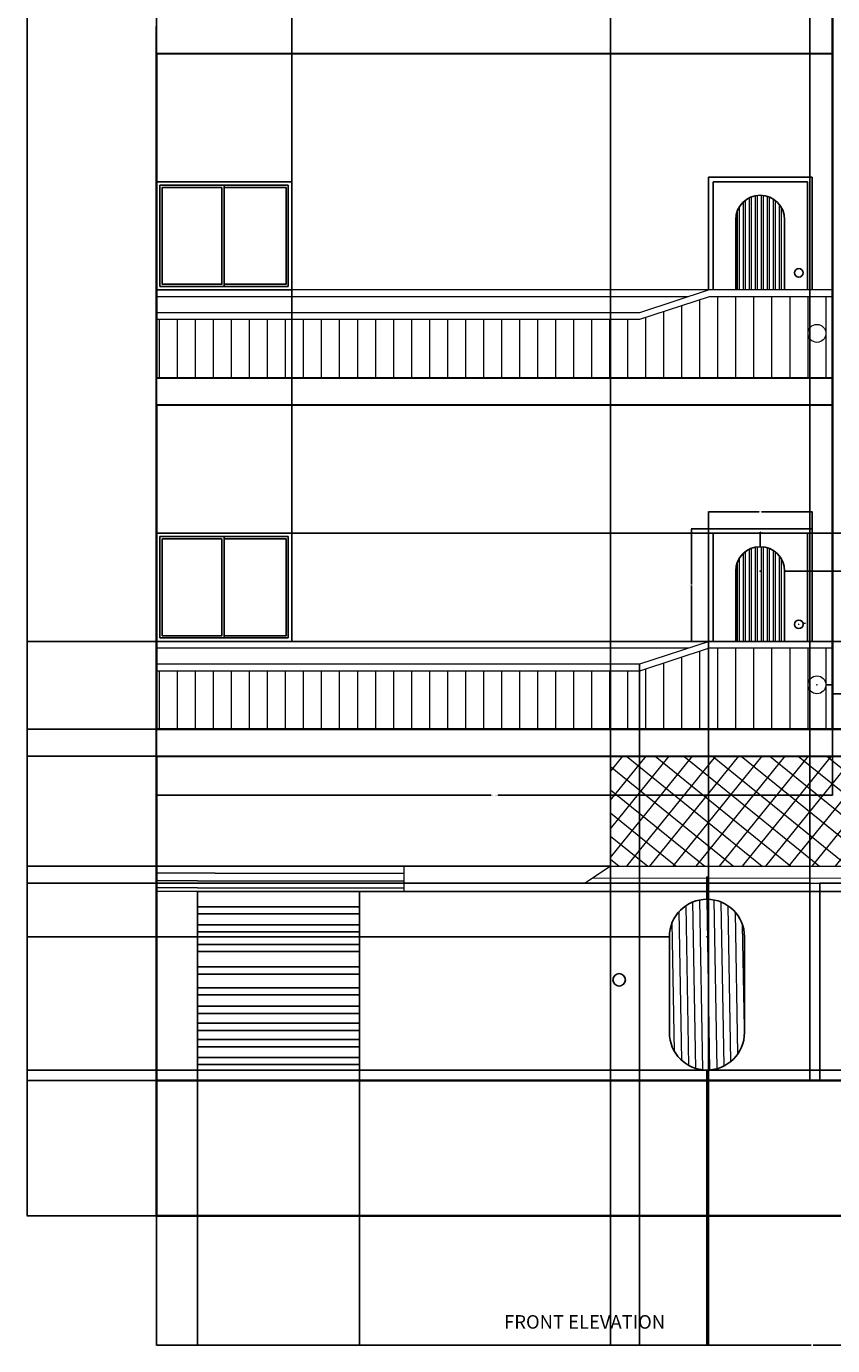
# Model space of a CAD drawing. Units: inches. Extents: x 373 to 969, y 157 to 1341.
# Tile 1 of 3: x 373 to 731, y 157 to 743. Entities that reach past the tile are written whole.
import ezdxf

# ---------------------------------------------------------------- set-up
doc = ezdxf.new("R2010")
doc.units = ezdxf.units.IN
doc.header["$MEASUREMENT"] = 0
for name, color, linetype, lineweight in [('A-ANNO-DIMS', 2, 'Continuous', 18), ('A-ANNO-TEXT', 7, 'Continuous', 25), ('A-DOOR', 3, 'Continuous', 25), ('A-DOOR-PATT', 8, 'Continuous', 13), ('A-ELEV-TRIM', 9, 'Continuous', 18), ('A-FLOR', 7, 'Continuous', 30), ('A-FLOR-HRAL', 4, 'Continuous', 18), ('A-FLOR-HRAL-PATT', 8, 'Continuous', 13), ('A-GLAZ', 4, 'Continuous', 25), ('A-WALL', 7, 'Continuous', 35), ('A-WALL-PATT', 8, 'Continuous', 13)]:
    doc.layers.add(name, color=color, linetype=linetype, lineweight=lineweight)
doc.styles.get("Standard").update_dxf_attribs({"font": 'arial.ttf'})
doc.dimstyles.get("Standard").update_dxf_attribs({"dimtxt": 0.18, "dimasz": 0.18, "dimexe": 0.18, "dimexo": 0.0625, "dimgap": 0.09, "dimtad": 0, "dimtih": 1, "dimtoh": 1, "dimdec": 4, "dimzin": 0, "dimdsep": 46, "dimlunit": 4, "dimtxsty": 'Standard', "dimcen": 0.09, "dimadec": 0, "dimazin": 0, "dimtfac": 1, "dimtdec": 4, "dimtofl": 0, "dimtmove": 0, "dimatfit": 3, "dimfxl": 1, "dimtolj": 1, "dimtzin": 0, "dimarcsym": 0})

# ---------------------------------------------------------------- blocks, each defined once
blk = doc.blocks.new('*U2')
for p, q in [((1.5, 1.5), (1.5, 46.5)), ((1.5, 46.5), (30, 46.5)), ((30, 1.5), (30, 46.5)), ((30, 46.5), (58.5, 46.5)), ((58.5, 46.5), (58.5, 1.5)), ((30, 1.5), (1.5, 1.5)), ((58.5, 1.5), (30, 1.5))]:
    blk.add_line(p, q)
blk.add_lwpolyline([(0, 0), (0, 48), (60, 48), (60, 0)], close=True)
for points in [[(29, 45.5), (29, 2.5), (2.5, 2.5), (2.5, 45.5), (29, 45.5)], [(30, 45.5), (57.5, 45.5), (57.5, 2.5), (30, 2.5)]]:
    blk.add_lwpolyline(points)
blk = doc.blocks.new('DOOR-ARCH-PANEL-ELEV')
for p, q in [((0, 48), (0, 50)), ((0, 50), (2, 50)), ((0, 48), (0, 0)), ((44, 50), (2, 50)), ((44, 48), (2, 48)), ((2, 48), (2, 0)), ((44, 50), (46, 50)), ((44, 0), (44, 48)), ((46, 50), (46, 48)), ((46, 0), (46, 48))]:
    blk.add_line(p, q)
for points in [[(12.07, 0), (12.07, 31.15)], [(33.78, 31.15), (33.78, 0)]]:
    blk.add_lwpolyline(points)
blk.add_circle((40.06, 7.56), 1.92)
blk.add_arc((22.93, 31.15), 10.86, 0, 180)
blk = doc.blocks.new('RAIL-BALCONY-SLOPED-ELEV')
for p, q in [((245.4, 23.26), (0, 23.26)), ((236.25, 20.26), (0, 20.26)), ((245.4, 23.26), (214.4, 13.09)), ((245.4, 20.26), (214.4, 10.09)), ((300.23, 23.26), (245.4, 23.26)), ((300.23, 20.26), (245.4, 20.26)), ((214.4, 13.09), (0, 13.09)), ((214.4, 10.09), (0, 10.09))]:
    blk.add_line(p, q)
blk.add_circle((293.27, 3.97), 3.97)
blk = doc.blocks.new('DOOR-OBROUND-INSERT-ELEV')
for points in [[(0, 16.68), (0, 59.13)], [(33.36, 59.13), (33.36, 16.68)]]:
    blk.add_lwpolyline(points)
for centre, start, end in [((16.68, 59.13), 0, 180), ((16.68, 16.68), 180, 0)]:
    blk.add_arc(centre, 16.68, start, end)
blk = doc.blocks.new('*D9')
at = {"layer": 'A-ANNO-DIMS', "color": 0, "lineweight": -2, "transparency": 16777216}
for p, q in [((675.76, 519.98), (668.14, 519.98)), ((668.32, 519.8), (668.32, 495.17)), ((668.32, 470.16), (668.32, 494.8)), ((675.76, 469.98), (668.14, 469.98))]:
    blk.add_line(p, q, dxfattribs=at)
at = {"layer": 'A-ANNO-DIMS', "color": 0, "transparency": 16777216}
for points in [[(668.29, 519.8), (668.35, 519.8), (668.32, 519.98)], [(668.29, 470.16), (668.35, 470.16), (668.32, 469.98)]]:
    blk.add_solid(points, dxfattribs=at)
at = {"layer": 'Defpoints', "color": 0, "transparency": 16777216}
for p in [(668.32, 519.98), (675.82, 519.98), (675.82, 469.98)]:
    blk.add_point(p, dxfattribs=at)
at = {"layer": 'A-ANNO-DIMS', "color": 0, "transparency": 16777216, "insert": (668.32, 494.98), "char_height": 0.18, "attachment_point": 5}
blk.add_mtext('\\A1;ARCH DOOR 50 TYP.', dxfattribs=at)
blk = doc.blocks.new('*D10')
at = {"layer": 'A-ANNO-DIMS', "color": 0, "lineweight": -2, "transparency": 16777216}
for p, q in [((675.82, 520.05), (675.82, 527.66)), ((676, 527.48), (698.29, 527.48)), ((721.64, 527.48), (699.36, 527.48)), ((721.82, 520.05), (721.82, 527.66))]:
    blk.add_line(p, q, dxfattribs=at)
at = {"layer": 'A-ANNO-DIMS', "color": 0, "transparency": 16777216}
for points in [[(676, 527.51), (676, 527.45), (675.82, 527.48)], [(721.64, 527.51), (721.64, 527.45), (721.82, 527.48)]]:
    blk.add_solid(points, dxfattribs=at)
at = {"layer": 'Defpoints', "color": 0, "transparency": 16777216}
for p in [(721.82, 527.48), (675.82, 519.98), (721.82, 519.98)]:
    blk.add_point(p, dxfattribs=at)
at = {"layer": 'A-ANNO-DIMS', "color": 0, "transparency": 16777216, "insert": (698.82, 527.48), "char_height": 0.18, "attachment_point": 5}
blk.add_mtext('\\A1;46 TYP.', dxfattribs=at)
blk = doc.blocks.new('*D11')
at = {"layer": 'A-ANNO-DIMS', "color": 0, "lineweight": -2, "transparency": 16777216}
for p, q in [((430.7, 446.66), (430.7, 401.51)), ((730.93, 446.66), (730.93, 401.51)), ((430.88, 401.69), (579.36, 401.69)), ((730.75, 401.69), (582.27, 401.69))]:
    blk.add_line(p, q, dxfattribs=at)
at = {"layer": 'A-ANNO-DIMS', "color": 0, "transparency": 16777216}
for points in [[(430.88, 401.72), (430.88, 401.66), (430.7, 401.69)], [(730.75, 401.72), (730.75, 401.66), (730.93, 401.69)]]:
    blk.add_solid(points, dxfattribs=at)
at = {"layer": 'Defpoints', "color": 0, "transparency": 16777216}
for p in [(430.7, 446.72), (730.93, 446.72), (730.93, 401.69)]:
    blk.add_point(p, dxfattribs=at)
at = {"layer": 'A-ANNO-DIMS', "color": 0, "transparency": 16777216, "insert": (580.82, 401.69), "char_height": 0.18, "attachment_point": 5}
blk.add_mtext('\\A1;SLOPED RAIL 300 TYP.', dxfattribs=at)
blk = doc.blocks.new('*D12')
at = {"layer": 'A-ANNO-DIMS', "color": 0, "lineweight": -2, "transparency": 16777216}
for p, q in [((731, 469.98), (776.15, 469.98)), ((775.97, 469.8), (775.97, 458.53)), ((775.97, 446.9), (775.97, 458.17)), ((731, 446.72), (776.15, 446.72))]:
    blk.add_line(p, q, dxfattribs=at)
at = {"layer": 'A-ANNO-DIMS', "color": 0, "transparency": 16777216}
for points in [[(775.94, 469.8), (776, 469.8), (775.97, 469.98)], [(775.94, 446.9), (776, 446.9), (775.97, 446.72)]]:
    blk.add_solid(points, dxfattribs=at)
at = {"layer": 'Defpoints', "color": 0, "transparency": 16777216}
for p in [(730.93, 469.98), (775.97, 469.98), (730.93, 446.72)]:
    blk.add_point(p, dxfattribs=at)
at = {"layer": 'A-ANNO-DIMS', "color": 0, "transparency": 16777216, "insert": (775.97, 458.35), "char_height": 0.18, "attachment_point": 5}
blk.add_mtext('\\A1;23 TYP.', dxfattribs=at)
blk = doc.blocks.new('*D27')
at = {"layer": 'A-ANNO-DIMS', "color": 0, "lineweight": -2, "transparency": 16777216}
for p, q in [((430.64, 469.98), (373.07, 469.98)), ((373.25, 469.8), (373.25, 450.67)), ((373.25, 431.16), (373.25, 450.3)), ((430.64, 430.98), (373.07, 430.98))]:
    blk.add_line(p, q, dxfattribs=at)
at = {"layer": 'A-ANNO-DIMS', "color": 0, "transparency": 16777216}
for points in [[(373.22, 469.8), (373.28, 469.8), (373.25, 469.98)], [(373.22, 431.16), (373.28, 431.16), (373.25, 430.98)]]:
    blk.add_solid(points, dxfattribs=at)
at = {"layer": 'Defpoints', "color": 0, "transparency": 16777216}
for p in [(373.25, 469.98), (430.7, 469.98), (430.7, 430.98)]:
    blk.add_point(p, dxfattribs=at)
at = {"layer": 'A-ANNO-DIMS', "color": 0, "transparency": 16777216, "insert": (373.25, 450.48), "char_height": 0.18, "attachment_point": 5}
blk.add_mtext('\\A1;39', dxfattribs=at)
blk = doc.blocks.new('*D28')
at = {"layer": 'A-ANNO-DIMS', "color": 0, "lineweight": -2, "transparency": 16777216}
for p, q in [((430.64, 430.98), (373.07, 430.98)), ((373.25, 430.8), (373.25, 425.16)), ((373.25, 419.16), (373.25, 424.8)), ((430.64, 418.98), (373.07, 418.98))]:
    blk.add_line(p, q, dxfattribs=at)
at = {"layer": 'A-ANNO-DIMS', "color": 0, "transparency": 16777216}
for points in [[(373.22, 430.8), (373.28, 430.8), (373.25, 430.98)], [(373.22, 419.16), (373.28, 419.16), (373.25, 418.98)]]:
    blk.add_solid(points, dxfattribs=at)
at = {"layer": 'Defpoints', "color": 0, "transparency": 16777216}
for p in [(373.25, 430.98), (430.7, 430.98), (430.7, 418.98)]:
    blk.add_point(p, dxfattribs=at)
at = {"layer": 'A-ANNO-DIMS', "color": 0, "transparency": 16777216, "insert": (373.25, 424.98), "char_height": 0.18, "attachment_point": 5}
blk.add_mtext('\\A1;12', dxfattribs=at)
blk = doc.blocks.new('*D29')
at = {"layer": 'A-ANNO-DIMS', "color": 0, "lineweight": -2, "transparency": 16777216}
for p, q in [((430.7, 518.05), (430.7, 1341.24)), ((490.7, 518.05), (490.7, 1341.24)), ((430.88, 1341.06), (460.48, 1341.06)), ((490.52, 1341.06), (460.92, 1341.06))]:
    blk.add_line(p, q, dxfattribs=at)
at = {"layer": 'A-ANNO-DIMS', "color": 0, "transparency": 16777216}
for points in [[(430.88, 1341.09), (430.88, 1341.03), (430.7, 1341.06)], [(490.52, 1341.09), (490.52, 1341.03), (490.7, 1341.06)]]:
    blk.add_solid(points, dxfattribs=at)
at = {"layer": 'Defpoints', "color": 0, "transparency": 16777216}
for p in [(490.7, 1341.06), (430.7, 517.98), (490.7, 517.98)]:
    blk.add_point(p, dxfattribs=at)
at = {"layer": 'A-ANNO-DIMS', "color": 0, "transparency": 16777216, "insert": (460.7, 1341.06), "char_height": 0.18, "attachment_point": 5}
blk.add_mtext('\\A1;60', dxfattribs=at)
blk = doc.blocks.new('*D30')
at = {"layer": 'A-ANNO-DIMS', "color": 0, "lineweight": -2, "transparency": 16777216}
for p, q in [((490.76, 517.98), (968.33, 517.98)), ((968.15, 517.8), (968.15, 494.17)), ((968.15, 470.16), (968.15, 493.8)), ((490.76, 469.98), (968.33, 469.98))]:
    blk.add_line(p, q, dxfattribs=at)
at = {"layer": 'A-ANNO-DIMS', "color": 0, "transparency": 16777216}
for points in [[(968.12, 517.8), (968.18, 517.8), (968.15, 517.98)], [(968.12, 470.16), (968.18, 470.16), (968.15, 469.98)]]:
    blk.add_solid(points, dxfattribs=at)
at = {"layer": 'Defpoints', "color": 0, "transparency": 16777216}
for p in [(490.7, 517.98), (968.15, 517.98), (490.7, 469.98)]:
    blk.add_point(p, dxfattribs=at)
at = {"layer": 'A-ANNO-DIMS', "color": 0, "transparency": 16777216, "insert": (968.15, 493.98), "char_height": 0.18, "attachment_point": 5}
blk.add_mtext('\\A1;48', dxfattribs=at)
blk = doc.blocks.new('*D31')
at = {"layer": 'A-ANNO-DIMS', "color": 0, "lineweight": -2, "transparency": 16777216}
for p, q in [((430.7, 459.75), (430.7, 157.35)), ((645.1, 459.75), (645.1, 157.35)), ((430.88, 157.53), (537.5, 157.53)), ((644.92, 157.53), (538.29, 157.53))]:
    blk.add_line(p, q, dxfattribs=at)
at = {"layer": 'A-ANNO-DIMS', "color": 0, "transparency": 16777216}
for points in [[(430.88, 157.56), (430.88, 157.5), (430.7, 157.53)], [(644.92, 157.56), (644.92, 157.5), (645.1, 157.53)]]:
    blk.add_solid(points, dxfattribs=at)
at = {"layer": 'Defpoints', "color": 0, "transparency": 16777216}
for p in [(430.7, 459.81), (645.1, 459.81), (645.1, 157.53)]:
    blk.add_point(p, dxfattribs=at)
at = {"layer": 'A-ANNO-DIMS', "color": 0, "transparency": 16777216, "insert": (537.9, 157.53), "char_height": 0.18, "attachment_point": 5}
blk.add_mtext('\\A1;214.4', dxfattribs=at)
blk = doc.blocks.new('*D32')
at = {"layer": 'A-ANNO-DIMS', "color": 0, "lineweight": -2, "transparency": 16777216}
for p, q in [((675.82, 469.92), (675.82, 157.35)), ((645.1, 459.75), (645.1, 157.35)), ((645.28, 157.53), (660, 157.53)), ((675.64, 157.53), (660.92, 157.53))]:
    blk.add_line(p, q, dxfattribs=at)
at = {"layer": 'A-ANNO-DIMS', "color": 0, "transparency": 16777216}
for points in [[(645.28, 157.56), (645.28, 157.5), (645.1, 157.53)], [(675.64, 157.56), (675.64, 157.5), (675.82, 157.53)]]:
    blk.add_solid(points, dxfattribs=at)
at = {"layer": 'Defpoints', "color": 0, "transparency": 16777216}
for p in [(675.82, 469.98), (645.1, 459.81), (675.82, 157.53)]:
    blk.add_point(p, dxfattribs=at)
at = {"layer": 'A-ANNO-DIMS', "color": 0, "transparency": 16777216, "insert": (660.46, 157.53), "char_height": 0.18, "attachment_point": 5}
blk.add_mtext('\\A1;30.726', dxfattribs=at)
blk = doc.blocks.new('*D33')
at = {"layer": 'A-ANNO-DIMS', "color": 0, "lineweight": -2, "transparency": 16777216}
for p, q in [((430.7, 274.92), (430.7, 157.35)), ((448.8, 274.92), (448.8, 157.35)), ((430.88, 157.53), (439.3, 157.53)), ((448.62, 157.53), (440.21, 157.53))]:
    blk.add_line(p, q, dxfattribs=at)
at = {"layer": 'A-ANNO-DIMS', "color": 0, "transparency": 16777216}
for points in [[(430.88, 157.56), (430.88, 157.5), (430.7, 157.53)], [(448.62, 157.56), (448.62, 157.5), (448.8, 157.53)]]:
    blk.add_solid(points, dxfattribs=at)
at = {"layer": 'Defpoints', "color": 0, "transparency": 16777216}
for p in [(430.7, 274.98), (448.8, 274.98), (448.8, 157.53)]:
    blk.add_point(p, dxfattribs=at)
at = {"layer": 'A-ANNO-DIMS', "color": 0, "transparency": 16777216, "insert": (439.75, 157.53), "char_height": 0.18, "attachment_point": 5}
blk.add_mtext('\\A1;18.103', dxfattribs=at)
blk = doc.blocks.new('*D34')
at = {"layer": 'A-ANNO-DIMS', "color": 0, "lineweight": -2, "transparency": 16777216}
for p, q in [((448.8, 274.92), (448.8, 157.35)), ((520.8, 274.92), (520.8, 157.35)), ((448.98, 157.53), (484.59, 157.53)), ((520.62, 157.53), (485.02, 157.53))]:
    blk.add_line(p, q, dxfattribs=at)
at = {"layer": 'A-ANNO-DIMS', "color": 0, "transparency": 16777216}
for points in [[(448.98, 157.56), (448.98, 157.5), (448.8, 157.53)], [(520.62, 157.56), (520.62, 157.5), (520.8, 157.53)]]:
    blk.add_solid(points, dxfattribs=at)
at = {"layer": 'Defpoints', "color": 0, "transparency": 16777216}
for p in [(448.8, 274.98), (520.8, 274.98), (520.8, 157.53)]:
    blk.add_point(p, dxfattribs=at)
at = {"layer": 'A-ANNO-DIMS', "color": 0, "transparency": 16777216, "insert": (484.8, 157.53), "char_height": 0.18, "attachment_point": 5}
blk.add_mtext('\\A1;72', dxfattribs=at)
blk = doc.blocks.new('*D35')
at = {"layer": 'A-ANNO-DIMS', "color": 0, "lineweight": -2, "transparency": 16777216}
for p, q in [((520.86, 358.98), (968.33, 358.98)), ((968.15, 358.8), (968.15, 317.17)), ((968.15, 275.16), (968.15, 316.8)), ((520.86, 274.98), (968.33, 274.98))]:
    blk.add_line(p, q, dxfattribs=at)
at = {"layer": 'A-ANNO-DIMS', "color": 0, "transparency": 16777216}
for points in [[(968.12, 358.8), (968.18, 358.8), (968.15, 358.98)], [(968.12, 275.16), (968.18, 275.16), (968.15, 274.98)]]:
    blk.add_solid(points, dxfattribs=at)
at = {"layer": 'Defpoints', "color": 0, "transparency": 16777216}
for p in [(520.8, 358.98), (968.15, 358.98), (520.8, 274.98)]:
    blk.add_point(p, dxfattribs=at)
at = {"layer": 'A-ANNO-DIMS', "color": 0, "transparency": 16777216, "insert": (968.15, 316.98), "char_height": 0.18, "attachment_point": 5}
blk.add_mtext('\\A1;84', dxfattribs=at)
blk = doc.blocks.new('*D36')
at = {"layer": 'A-ANNO-DIMS', "color": 0, "lineweight": -2, "transparency": 16777216}
for p, q in [((520.8, 274.92), (520.8, 157.35)), ((632.3, 274.92), (632.3, 157.35)), ((520.98, 157.53), (576.17, 157.53)), ((632.12, 157.53), (576.94, 157.53))]:
    blk.add_line(p, q, dxfattribs=at)
at = {"layer": 'A-ANNO-DIMS', "color": 0, "transparency": 16777216}
for points in [[(520.98, 157.56), (520.98, 157.5), (520.8, 157.53)], [(632.12, 157.56), (632.12, 157.5), (632.3, 157.53)]]:
    blk.add_solid(points, dxfattribs=at)
at = {"layer": 'Defpoints', "color": 0, "transparency": 16777216}
for p in [(520.8, 274.98), (632.3, 274.98), (632.3, 157.53)]:
    blk.add_point(p, dxfattribs=at)
at = {"layer": 'A-ANNO-DIMS', "color": 0, "transparency": 16777216, "insert": (576.55, 157.53), "char_height": 0.18, "attachment_point": 5}
blk.add_mtext('\\A1;111.5', dxfattribs=at)
blk = doc.blocks.new('*D37')
at = {"layer": 'A-ANNO-DIMS', "color": 0, "lineweight": -2, "transparency": 16777216}
for p, q in [((632.24, 362.6), (373.07, 362.6)), ((373.25, 362.42), (373.25, 318.98)), ((373.25, 275.16), (373.25, 318.61)), ((632.24, 274.98), (373.07, 274.98))]:
    blk.add_line(p, q, dxfattribs=at)
at = {"layer": 'A-ANNO-DIMS', "color": 0, "transparency": 16777216}
for points in [[(373.22, 362.42), (373.28, 362.42), (373.25, 362.6)], [(373.22, 275.16), (373.28, 275.16), (373.25, 274.98)]]:
    blk.add_solid(points, dxfattribs=at)
at = {"layer": 'Defpoints', "color": 0, "transparency": 16777216}
for p in [(373.25, 362.6), (632.3, 362.6), (632.3, 274.98)]:
    blk.add_point(p, dxfattribs=at)
at = {"layer": 'A-ANNO-DIMS', "color": 0, "transparency": 16777216, "insert": (373.25, 318.79), "char_height": 0.18, "attachment_point": 5}
blk.add_mtext('\\A1;87.62', dxfattribs=at)
blk = doc.blocks.new('*D38')
at = {"layer": 'A-ANNO-DIMS', "color": 0, "lineweight": -2, "transparency": 16777216}
for p, q in [((632.26, 418.98), (373.07, 418.98)), ((373.25, 418.8), (373.25, 394.78)), ((373.25, 370.39), (373.25, 394.41)), ((632.26, 370.21), (373.07, 370.21))]:
    blk.add_line(p, q, dxfattribs=at)
at = {"layer": 'A-ANNO-DIMS', "color": 0, "transparency": 16777216}
for points in [[(373.22, 418.8), (373.28, 418.8), (373.25, 418.98)], [(373.22, 370.39), (373.28, 370.39), (373.25, 370.21)]]:
    blk.add_solid(points, dxfattribs=at)
at = {"layer": 'Defpoints', "color": 0, "transparency": 16777216}
for p in [(373.25, 418.98), (632.32, 418.98), (632.32, 370.21)]:
    blk.add_point(p, dxfattribs=at)
at = {"layer": 'A-ANNO-DIMS', "color": 0, "transparency": 16777216, "insert": (373.25, 394.6), "char_height": 0.18, "attachment_point": 5}
blk.add_mtext('\\A1;48.78', dxfattribs=at)
blk = doc.blocks.new('*D39')
at = {"layer": 'A-ANNO-DIMS', "color": 0, "lineweight": -2, "transparency": 16777216}
for p, q in [((675.1, 279.62), (675.1, 157.35)), ((632.3, 274.92), (632.3, 157.35)), ((632.48, 157.53), (653.37, 157.53)), ((674.92, 157.53), (654.03, 157.53))]:
    blk.add_line(p, q, dxfattribs=at)
at = {"layer": 'A-ANNO-DIMS', "color": 0, "transparency": 16777216}
for points in [[(632.48, 157.56), (632.48, 157.5), (632.3, 157.53)], [(674.92, 157.56), (674.92, 157.5), (675.1, 157.53)]]:
    blk.add_solid(points, dxfattribs=at)
at = {"layer": 'Defpoints', "color": 0, "transparency": 16777216}
for p in [(675.1, 279.69), (632.3, 274.98), (675.1, 157.53)]:
    blk.add_point(p, dxfattribs=at)
at = {"layer": 'A-ANNO-DIMS', "color": 0, "transparency": 16777216, "insert": (653.7, 157.53), "char_height": 0.18, "attachment_point": 5}
blk.add_mtext('\\A1;42.8', dxfattribs=at)
blk = doc.blocks.new('*D40')
at = {"layer": 'A-ANNO-DIMS', "color": 0, "lineweight": -2, "transparency": 16777216}
for p, q in [((675.1, 279.62), (675.1, 157.35)), ((768.63, 279.62), (768.63, 157.35)), ((675.28, 157.53), (721.47, 157.53)), ((768.45, 157.53), (722.26, 157.53))]:
    blk.add_line(p, q, dxfattribs=at)
at = {"layer": 'A-ANNO-DIMS', "color": 0, "transparency": 16777216}
for points in [[(675.28, 157.56), (675.28, 157.5), (675.1, 157.53)], [(768.45, 157.56), (768.45, 157.5), (768.63, 157.53)]]:
    blk.add_solid(points, dxfattribs=at)
at = {"layer": 'Defpoints', "color": 0, "transparency": 16777216}
for p in [(675.1, 279.69), (768.63, 279.69), (768.63, 157.53)]:
    blk.add_point(p, dxfattribs=at)
at = {"layer": 'A-ANNO-DIMS', "color": 0, "transparency": 16777216, "insert": (721.86, 157.53), "char_height": 0.18, "attachment_point": 5}
blk.add_mtext('\\A1;93.53', dxfattribs=at)
blk = doc.blocks.new('*D42')
at = {"layer": 'A-ANNO-DIMS', "color": 0, "lineweight": -2, "transparency": 16777216}
for p, q in [((632.3, 362.67), (632.3, 1341.24)), ((720.88, 362.67), (720.88, 1341.24)), ((632.48, 1341.06), (676.2, 1341.06)), ((720.7, 1341.06), (676.98, 1341.06))]:
    blk.add_line(p, q, dxfattribs=at)
at = {"layer": 'A-ANNO-DIMS', "color": 0, "transparency": 16777216}
for points in [[(632.48, 1341.09), (632.48, 1341.03), (632.3, 1341.06)], [(720.7, 1341.09), (720.7, 1341.03), (720.88, 1341.06)]]:
    blk.add_solid(points, dxfattribs=at)
at = {"layer": 'Defpoints', "color": 0, "transparency": 16777216}
for p in [(720.88, 1341.06), (632.3, 362.6), (720.88, 362.6)]:
    blk.add_point(p, dxfattribs=at)
at = {"layer": 'A-ANNO-DIMS', "color": 0, "transparency": 16777216, "insert": (676.59, 1341.06), "char_height": 0.18, "attachment_point": 5}
blk.add_mtext('\\A1;88.58', dxfattribs=at)
blk = doc.blocks.new('*D43')
at = {"layer": 'A-ANNO-DIMS', "color": 0, "lineweight": -2, "transparency": 16777216}
for p, q in [((658.36, 338.82), (373.07, 338.82)), ((373.25, 338.64), (373.25, 309.43)), ((373.25, 279.87), (373.25, 309.07)), ((675.03, 279.69), (373.07, 279.69))]:
    blk.add_line(p, q, dxfattribs=at)
at = {"layer": 'A-ANNO-DIMS', "color": 0, "transparency": 16777216}
for points in [[(373.22, 338.64), (373.28, 338.64), (373.25, 338.82)], [(373.22, 279.87), (373.28, 279.87), (373.25, 279.69)]]:
    blk.add_solid(points, dxfattribs=at)
at = {"layer": 'Defpoints', "color": 0, "transparency": 16777216}
for p in [(373.25, 338.82), (658.42, 338.82), (675.1, 279.69)]:
    blk.add_point(p, dxfattribs=at)
at = {"layer": 'A-ANNO-DIMS', "color": 0, "transparency": 16777216, "insert": (373.25, 309.25), "char_height": 0.18, "attachment_point": 5}
blk.add_mtext('\\A1;59.13', dxfattribs=at)
blk = doc.blocks.new('*D44')
at = {"layer": 'A-ANNO-DIMS', "color": 0, "lineweight": -2, "transparency": 16777216}
for p, q in [((860.91, 279.69), (373.07, 279.69)), ((373.25, 279.51), (373.25, 277.52)), ((373.25, 275.16), (373.25, 277.15)), ((818.75, 274.98), (373.07, 274.98))]:
    blk.add_line(p, q, dxfattribs=at)
at = {"layer": 'A-ANNO-DIMS', "color": 0, "transparency": 16777216}
for points in [[(373.22, 279.51), (373.28, 279.51), (373.25, 279.69)], [(373.22, 275.16), (373.28, 275.16), (373.25, 274.98)]]:
    blk.add_solid(points, dxfattribs=at)
at = {"layer": 'Defpoints', "color": 0, "transparency": 16777216}
for p in [(373.25, 279.69), (860.97, 279.69), (818.82, 274.98)]:
    blk.add_point(p, dxfattribs=at)
at = {"layer": 'A-ANNO-DIMS', "color": 0, "transparency": 16777216, "insert": (373.25, 277.34), "char_height": 0.18, "attachment_point": 5}
blk.add_mtext('\\A1;4.702', dxfattribs=at)
blk = doc.blocks.new('*D45')
at = {"layer": 'A-ANNO-DIMS', "color": 0, "lineweight": -2, "transparency": 16777216}
for p, q in [((709.67, 501.13), (968.33, 501.13)), ((968.15, 500.95), (968.15, 485.74)), ((968.15, 470.16), (968.15, 485.38)), ((721.89, 469.98), (968.33, 469.98))]:
    blk.add_line(p, q, dxfattribs=at)
at = {"layer": 'A-ANNO-DIMS', "color": 0, "transparency": 16777216}
for points in [[(968.12, 500.95), (968.18, 500.95), (968.15, 501.13)], [(968.12, 470.16), (968.18, 470.16), (968.15, 469.98)]]:
    blk.add_solid(points, dxfattribs=at)
at = {"layer": 'Defpoints', "color": 0, "transparency": 16777216}
for p in [(709.61, 501.13), (968.15, 501.13), (721.82, 469.98)]:
    blk.add_point(p, dxfattribs=at)
at = {"layer": 'A-ANNO-DIMS', "color": 0, "transparency": 16777216, "insert": (968.15, 485.56), "char_height": 0.18, "attachment_point": 5}
blk.add_mtext('\\A1;31.146', dxfattribs=at)
blk = doc.blocks.new('*D55')
at = {"layer": 'A-ANNO-DIMS', "color": 0, "lineweight": -2, "transparency": 16777216}
for p, q in [((734.58, 1283.61), (373.07, 1283.61)), ((373.25, 1283.43), (373.25, 749.48)), ((373.25, 215.16), (373.25, 749.11)), ((430.64, 214.98), (373.07, 214.98))]:
    blk.add_line(p, q, dxfattribs=at)
at = {"layer": 'A-ANNO-DIMS', "color": 0, "transparency": 16777216}
for points in [[(373.22, 1283.43), (373.28, 1283.43), (373.25, 1283.61)], [(373.22, 215.16), (373.28, 215.16), (373.25, 214.98)]]:
    blk.add_solid(points, dxfattribs=at)
at = {"layer": 'Defpoints', "color": 0, "transparency": 16777216}
for p in [(373.25, 1283.61), (734.64, 1283.61), (430.7, 214.98)]:
    blk.add_point(p, dxfattribs=at)
at = {"layer": 'A-ANNO-DIMS', "color": 0, "transparency": 16777216, "insert": (373.25, 749.3), "char_height": 0.18, "attachment_point": 5}
blk.add_mtext('\\A1;1068.6', dxfattribs=at)
blk = doc.blocks.new('*D56')
at = {"layer": 'A-ANNO-DIMS', "color": 0, "lineweight": -2, "transparency": 16777216}
for p, q in [((675.28, 365.5), (675.1, 365.5)), ((675.1, 365.5), (675.1, 355.67)), ((675.01, 338.82), (675.19, 338.82)), ((675.1, 338.73), (675.1, 338.91))]:
    blk.add_line(p, q, dxfattribs=at)
at = {"layer": 'A-ANNO-DIMS', "color": 0, "transparency": 16777216}
blk.add_solid([(675.07, 355.67), (675.13, 355.67), (675.1, 355.49)], dxfattribs=at)
at = {"layer": 'Defpoints', "color": 0, "transparency": 16777216}
for p in [(675.1, 355.49), (675.1, 338.82)]:
    blk.add_point(p, dxfattribs=at)
at = {"layer": 'A-ANNO-DIMS', "color": 0, "transparency": 16777216, "insert": (676.02, 365.5), "char_height": 0.18, "attachment_point": 5}
blk.add_mtext('\\A1;6X R16.678', dxfattribs=at)
blk = doc.blocks.new('*D57')
at = {"layer": 'A-ANNO-DIMS', "color": 0, "lineweight": -2, "transparency": 16777216}
for p, q in [((698.93, 518.5), (698.75, 518.5)), ((698.75, 518.5), (698.75, 512.17)), ((698.66, 501.13), (698.84, 501.13)), ((698.75, 501.04), (698.75, 501.22))]:
    blk.add_line(p, q, dxfattribs=at)
at = {"layer": 'A-ANNO-DIMS', "color": 0, "transparency": 16777216}
blk.add_solid([(698.72, 512.17), (698.78, 512.17), (698.75, 511.99)], dxfattribs=at)
at = {"layer": 'Defpoints', "color": 0, "transparency": 16777216}
for p in [(698.75, 511.99), (698.75, 501.13)]:
    blk.add_point(p, dxfattribs=at)
at = {"layer": 'A-ANNO-DIMS', "color": 0, "transparency": 16777216, "insert": (699.68, 518.5), "char_height": 0.18, "attachment_point": 5}
blk.add_mtext('\\A1;4X R10.855', dxfattribs=at)
blk = doc.blocks.new('*D58')
at = {"layer": 'A-ANNO-DIMS', "color": 0, "lineweight": -2, "transparency": 16777216}
for p, q in [((723.88, 450.69), (724.06, 450.69)), ((723.97, 450.6), (723.97, 450.78)), ((730.33, 450.7), (728.12, 450.7))]:
    blk.add_line(p, q, dxfattribs=at)
at = {"layer": 'A-ANNO-DIMS', "color": 0, "transparency": 16777216}
blk.add_solid([(728.12, 450.73), (728.12, 450.67), (727.94, 450.7)], dxfattribs=at)
at = {"layer": 'Defpoints', "color": 0, "transparency": 16777216}
for p in [(720, 450.69), (727.94, 450.7)]:
    blk.add_point(p, dxfattribs=at)
at = {"layer": 'A-ANNO-DIMS', "color": 0, "transparency": 16777216, "insert": (731.01, 450.7), "char_height": 0.18, "attachment_point": 5}
blk.add_mtext('\\A1;4X ∅7.946', dxfattribs=at)
blk = doc.blocks.new('*D59')
at = {"layer": 'A-ANNO-DIMS', "color": 0, "lineweight": -2, "transparency": 16777216}
for p, q in [((715.79, 477.55), (715.97, 477.55)), ((715.88, 477.46), (715.88, 477.64)), ((718.9, 478.13), (717.94, 477.95))]:
    blk.add_line(p, q, dxfattribs=at)
at = {"layer": 'A-ANNO-DIMS', "color": 0, "transparency": 16777216}
blk.add_solid([(717.94, 477.98), (717.95, 477.92), (717.76, 477.91)], dxfattribs=at)
at = {"layer": 'Defpoints', "color": 0, "transparency": 16777216}
for p in [(713.99, 477.18), (717.76, 477.91)]:
    blk.add_point(p, dxfattribs=at)
at = {"layer": 'A-ANNO-DIMS', "color": 0, "transparency": 16777216, "insert": (719.58, 478.13), "char_height": 0.18, "attachment_point": 5}
blk.add_mtext('\\A1;4X ∅3.842', dxfattribs=at)

msp = doc.modelspace()

# ---------------------------------------------------------------- hatches: boundary and pattern name
at = {"layer": 'A-DOOR-PATT'}
h = msp.add_hatch(dxfattribs=at)
h.set_pattern_fill('ANSI32', color=256, scale=7.1, angle=225)
h.set_pattern_definition([(270, (0, 156), (2.6625, -4e-16), []), (270, (-0.8875, 155.1125), (2.6625, -4e-16), [])])
h.paths.add_polyline_path([(709.6057, 657.1302, 1), (687.8953, 657.1302), (687.8953, 625.9843), (709.6057, 625.9843)])
h = msp.add_hatch(dxfattribs=at)
h.set_pattern_fill('ANSI32', color=256, scale=7.1, angle=225)
h.paths.add_polyline_path([(709.6057, 501.1302, 1), (687.8953, 501.1302), (687.8953, 469.9843), (709.6057, 469.9843)])
h = msp.add_hatch(dxfattribs=at)
h.set_pattern_fill('ANSI31', color=256, scale=25, angle=226)
h.paths.add_polyline_path([(691.7746, 338.8165, 1), (658.4191, 338.8165), (658.4191, 296.364, 1), (691.7746, 296.364)])
at = {"layer": 'A-FLOR-HRAL-PATT'}
h = msp.add_hatch(dxfattribs=at)
h.set_pattern_fill('ANSI31', color=256, scale=64, angle=225)
h.set_pattern_definition([(270, (0, 156), (8, -9e-16), [])])
h.paths.add_polyline_path([(730.9335, 622.9843), (676.0953, 622.9843), (645.0983, 612.8114), (430.6998, 612.8114), (430.6998, 586.9843), (730.9335, 586.9843)])
h = msp.add_hatch(dxfattribs=at)
h.set_pattern_fill('ANSI31', color=256, scale=64, angle=225)
h.paths.add_polyline_path([(430.6998, 456.8114), (430.6998, 430.9843), (730.9335, 430.9843), (730.9335, 466.9843), (676.0953, 466.9843), (645.0983, 456.8114)])
at = {"layer": 'A-WALL-PATT'}
h = msp.add_hatch(dxfattribs=at)
h.set_pattern_fill('ANSI37', color=256, scale=64, angle=96)
h.paths.add_polyline_path([(903.5487, 418.9843), (632.3184, 418.9843), (632.3184, 370.2071), (903.5487, 370.2071)])

# ---------------------------------------------------------------- linework, layer by layer
at = {"layer": 'A-DOOR'}
for p, q in [((448.8024, 274.9843), (448.8024, 358.9843)), ((448.8024, 358.9843), (520.8024, 358.9843)), ((520.8024, 358.9843), (520.8024, 274.9843)), ((448.8024, 352.1648), (520.8024, 352.1648)), ((448.8024, 348.9982), (520.8024, 348.9982)), ((448.8024, 344.2038), (520.8024, 344.2038)), ((448.8024, 341.0372), (520.8024, 341.0372)), ((448.8024, 335.4709), (520.8024, 335.4709)), ((448.8024, 332.3043), (520.8024, 332.3043)), ((448.8024, 325.4835), (520.8024, 325.4835)), ((448.8024, 322.3169), (520.8024, 322.3169)), ((448.8024, 316.2198), (520.8024, 316.2198)), ((448.8024, 313.0532), (520.8024, 313.0532)), ((448.8024, 307.9694), (520.8024, 307.9694)), ((448.8024, 304.8028), (520.8024, 304.8028)), ((448.8024, 300.4426), (520.8024, 300.4426)), ((448.8024, 297.276), (520.8024, 297.276)), ((448.8024, 293.2054), (520.8024, 293.2054)), ((448.8024, 290.0388), (520.8024, 290.0388)), ((448.8024, 285.2592), (520.8024, 285.2592)), ((448.8024, 282.0926), (520.8024, 282.0926))]:
    msp.add_line(p, q, dxfattribs=at)
for points in [[(632.3006, 362.6044), (720.8808, 362.6044), (720.8808, 274.9843), (632.3006, 274.9843)], [(725.2573, 362.6044), (813.8375, 362.6044), (813.8375, 274.9843), (725.2573, 274.9843)]]:
    msp.add_lwpolyline(points, close=True, dxfattribs=at)
msp.add_circle((636.1365, 319.7202), 2.7765, dxfattribs=at)
at = {"layer": 'A-ELEV-TRIM'}
for p, q in [((632.3184, 418.9843), (632.3184, 370.2071)), ((430.6998, 358.9843), (430.6998, 370.2071)), ((430.6998, 370.2071), (540.4426, 370.2071)), ((540.4426, 370.2071), (540.4426, 358.9843)), ((632.3184, 370.2071), (620.9782, 362.6044)), ((632.3184, 370.2071), (903.5487, 370.2071)), ((456.7424, 367.0405), (430.6998, 367.0405)), ((448.8024, 363.7444), (430.6998, 363.7444)), ((448.8024, 363.7444), (520.8024, 363.7444)), ((456.7424, 367.0405), (528.7424, 367.0405)), ((520.8024, 363.7444), (540.4426, 363.7444)), ((528.7424, 367.0405), (540.4426, 367.0405)), ((624.5243, 364.9818), (908.76, 364.6667)), ((448.8024, 360.5778), (430.6998, 360.5778)), ((448.8024, 358.9843), (430.6998, 358.9843)), ((448.8024, 360.5778), (520.8024, 360.5778)), ((520.8024, 360.5778), (540.4426, 360.5778)), ((540.4426, 358.9843), (520.8024, 358.9843)), ((620.9782, 362.6044), (910.6998, 362.6044))]:
    msp.add_line(p, q, dxfattribs=at)
at = {"layer": 'A-FLOR'}
for p, q in [((430.6998, 730.9843), (430.6998, 742.9843)), ((430.6998, 730.9843), (730.9335, 730.9843)), ((430.6998, 574.9843), (430.6998, 586.9843)), ((430.6998, 586.9843), (730.9335, 586.9843)), ((430.6998, 574.9843), (730.9335, 574.9843)), ((430.6998, 418.9843), (430.6998, 430.9843)), ((430.6998, 418.9843), (910.6998, 418.9843))]:
    msp.add_line(p, q, dxfattribs=at)
at = {"layer": 'A-FLOR-HRAL'}
msp.add_line((730.9335, 430.9843), (730.9335, 466.9843), dxfattribs=at)
at = {"layer": 'A-WALL'}
for p, q in [((730.9335, 587.7283), (730.9335, 856.4498)), ((430.6998, 586.9843), (430.6998, 730.9843)), ((730.9335, 587.7283), (730.9335, 430.9843)), ((430.6998, 430.9843), (430.6998, 574.9843)), ((430.6998, 274.9843), (430.6998, 418.9843)), ((910.6998, 274.9843), (430.6998, 274.9843)), ((430.6998, 274.9843), (430.6998, 214.9843)), ((430.6998, 214.9843), (910.6998, 214.9843))]:
    msp.add_line(p, q, dxfattribs=at)
msp.add_lwpolyline([(430.6998, 430.9843), (910.6998, 430.9843), (910.6998, 1276.1757)], dxfattribs=at)

# ---------------------------------------------------------------- block references
at = {"layer": 'A-DOOR'}
for name, p in [('DOOR-ARCH-PANEL-ELEV', (675.824, 625.984)), ('DOOR-ARCH-PANEL-ELEV', (675.824, 469.984)), ('DOOR-OBROUND-INSERT-ELEV', (658.419, 279.686))]:
    msp.add_blockref(name, p, dxfattribs=at)
at = {"layer": 'A-FLOR-HRAL'}
for p in [(430.7, 602.722), (430.7, 446.722)]:
    msp.add_blockref('RAIL-BALCONY-SLOPED-ELEV', p, dxfattribs=at)
at = {"layer": 'A-GLAZ'}
for p in [(430.6998, 625.9843), (430.6998, 469.9843)]:
    msp.add_blockref('*U2', p, dxfattribs=at)

# ---------------------------------------------------------------- texts
at = {"layer": 'A-ANNO-TEXT', "insert": (585.0365, 170.8821), "char_height": 6, "attachment_point": 1}
msp.add_mtext_dynamic_manual_height_columns('FRONT ELEVATION', width=212.774286, gutter_width=1, heights=[0], dxfattribs=at)

# ---------------------------------------------------------------- dimensions: what is measured, and where the dimension line sits
at = {"layer": 'A-ANNO-DIMS'}
for base, p1, p2, override, picture, middle in [((490.6998, 1341.0564), (430.6998, 517.9843), (490.6998, 517.9843), {"dimdec": 0, "dimlfac": 1, "dimrnd": 0, "dimzin": 0, "dimdsep": 46, "dimlunit": 2}, '*D29', (460.6998, 1341.0564)), ((720.8808, 1341.0564), (632.3006, 362.6044), (720.8808, 362.6044), {"dimdec": 2, "dimlfac": 1, "dimrnd": 0, "dimzin": 0, "dimdsep": 46, "dimlunit": 2}, '*D42', (676.5907, 1341.0564)), ((675.8241, 157.5343), (645.0983, 459.8114), (675.8241, 469.9843), {"dimdec": 3, "dimlfac": 1, "dimrnd": 0, "dimzin": 0, "dimdsep": 46, "dimlunit": 2}, '*D32', (660.4612, 157.5343)), ((645.0983, 157.5343), (430.6998, 459.8114), (645.0983, 459.8114), {"dimdec": 1, "dimlfac": 1, "dimrnd": 0, "dimzin": 0, "dimdsep": 46, "dimlunit": 2}, '*D31', (537.8991, 157.5343)), ((675.0969, 157.5343), (632.3006, 274.9843), (675.0969, 279.6862), {"dimdec": 1, "dimlfac": 1, "dimrnd": 0, "dimzin": 0, "dimdsep": 46, "dimlunit": 2}, '*D39', (653.6987, 157.5343)), ((768.6299, 157.5343), (675.0969, 279.6862), (768.6299, 279.6862), {"dimdec": 2, "dimlfac": 1, "dimrnd": 0, "dimzin": 0, "dimdsep": 46, "dimlunit": 2}, '*D40', (721.8634, 157.5343)), ((448.8024, 157.5343), (430.6998, 274.9843), (448.8024, 274.9843), {"dimdec": 3, "dimlfac": 1, "dimrnd": 0, "dimzin": 0, "dimdsep": 46, "dimlunit": 2}, '*D33', (439.7511, 157.5343)), ((520.8024, 157.5343), (448.8024, 274.9843), (520.8024, 274.9843), {"dimdec": 0, "dimlfac": 1, "dimrnd": 0, "dimzin": 0, "dimdsep": 46, "dimlunit": 2}, '*D34', (484.8024, 157.5343)), ((632.3006, 157.5343), (520.8024, 274.9843), (632.3006, 274.9843), {"dimdec": 1, "dimlfac": 1, "dimrnd": 0, "dimzin": 0, "dimdsep": 46, "dimlunit": 2}, '*D36', (576.5515, 157.5343))]:
    dim = msp.add_linear_dim(base=base, p1=p1, p2=p2, dimstyle='Standard', override=override, dxfattribs=at)
    dim.commit()
    dim.dimension.update_dxf_attribs({"geometry": picture, "text_midpoint": middle})
for base, p1, p2, override, picture, middle in [((373.2498, 1283.6064), (430.6998, 214.9843), (734.6424, 1283.6064), {"dimdec": 1, "dimlfac": 1, "dimrnd": 0, "dimzin": 0, "dimdsep": 46, "dimlunit": 2}, '*D55', (373.2498, 749.2954)), ((968.1498, 517.9843), (490.6998, 469.9843), (490.6998, 517.9843), {"dimdec": 0, "dimlfac": 1, "dimrnd": 0, "dimzin": 0, "dimdsep": 46, "dimlunit": 2}, '*D30', (968.1498, 493.9843)), ((968.1498, 501.1302), (721.8241, 469.9843), (709.6057, 501.1302), {"dimdec": 3, "dimlfac": 1, "dimrnd": 0, "dimzin": 0, "dimdsep": 46, "dimlunit": 2}, '*D45', (968.1498, 485.5573)), ((373.2498, 469.9843), (430.6998, 430.9843), (430.6998, 469.9843), {"dimdec": 0, "dimlfac": 1, "dimrnd": 0, "dimzin": 0, "dimdsep": 46, "dimlunit": 2}, '*D27', (373.2498, 450.4843)), ((373.2498, 430.9843), (430.6998, 418.9843), (430.6998, 430.9843), {"dimdec": 0, "dimlfac": 1, "dimrnd": 0, "dimzin": 0, "dimdsep": 46, "dimlunit": 2}, '*D28', (373.2498, 424.9843)), ((373.2498, 418.9843), (632.3184, 370.2071), (632.3184, 418.9843), {"dimdec": 2, "dimlfac": 1, "dimrnd": 0, "dimzin": 0, "dimdsep": 46, "dimlunit": 2}, '*D38', (373.2498, 394.5957)), ((373.2498, 362.6044), (632.3006, 274.9843), (632.3006, 362.6044), {"dimdec": 2, "dimlfac": 1, "dimrnd": 0, "dimzin": 0, "dimdsep": 46, "dimlunit": 2}, '*D37', (373.2498, 318.7943)), ((968.1498, 358.9843), (520.8024, 274.9843), (520.8024, 358.9843), {"dimdec": 0, "dimlfac": 1, "dimrnd": 0, "dimzin": 0, "dimdsep": 46, "dimlunit": 2}, '*D35', (968.1498, 316.9843)), ((373.2498, 338.8165), (675.0969, 279.6862), (658.4191, 338.8165), {"dimdec": 2, "dimlfac": 1, "dimrnd": 0, "dimzin": 0, "dimdsep": 46, "dimlunit": 2}, '*D43', (373.2498, 309.2514)), ((373.2498, 279.6862), (818.8151, 274.9843), (860.9749, 279.6862), {"dimdec": 3, "dimlfac": 1, "dimrnd": 0, "dimzin": 0, "dimdsep": 46, "dimlunit": 2}, '*D44', (373.2498, 277.3353))]:
    dim = msp.add_linear_dim(base=base, p1=p1, p2=p2, angle=90, dimstyle='Standard', override=override, dxfattribs=at)
    dim.commit()
    dim.dimension.update_dxf_attribs({"geometry": picture, "text_midpoint": middle})
for base, p1, p2, text, picture, middle in [((721.8241, 527.4843), (675.8241, 519.9843), (721.8241, 519.9843), '<> TYP.', '*D10', (698.8241, 527.4843)), ((730.9335, 401.6867), (430.6998, 446.7217), (730.9335, 446.7217), 'SLOPED RAIL <> TYP.', '*D11', (580.8166, 401.6867))]:
    dim = msp.add_linear_dim(base=base, p1=p1, p2=p2, text=text, dimstyle='Standard', override={"dimdec": 0, "dimlfac": 1, "dimrnd": 0, "dimzin": 0, "dimdsep": 46, "dimlunit": 2}, dxfattribs=at)
    dim.commit()
    dim.dimension.update_dxf_attribs({"geometry": picture, "text_midpoint": middle})
for base, p1, p2, text, picture, middle in [((668.3241, 519.9843), (675.8241, 469.9843), (675.8241, 519.9843), 'ARCH DOOR <> TYP.', '*D9', (668.3241, 494.9843)), ((775.9685, 469.9843), (730.9335, 446.7217), (730.9335, 469.9843), '<> TYP.', '*D12', (775.9685, 458.353))]:
    dim = msp.add_linear_dim(base=base, p1=p1, p2=p2, angle=90, text=text, dimstyle='Standard', override={"dimdec": 0, "dimlfac": 1, "dimrnd": 0, "dimzin": 0, "dimdsep": 46, "dimlunit": 2}, dxfattribs=at)
    dim.commit()
    dim.dimension.update_dxf_attribs({"geometry": picture, "text_midpoint": middle})
for center, mpoint, text, picture, middle in [((698.7505, 501.1302), (698.751, 511.9854), '4X <>', '*D57', (699.6787, 518.4986)), ((675.0969, 338.8165), (675.097, 355.4943), '6X <>', '*D56', (676.0209, 365.5009))]:
    dim = msp.add_radius_dim(center=center, mpoint=mpoint, text=text, dimstyle='Standard', override={"dimdec": 3, "dimlfac": 1, "dimrnd": 0, "dimzin": 0, "dimdsep": 46, "dimlunit": 2}, dxfattribs=at)
    dim.commit()
    dim.dimension.update_dxf_attribs({"geometry": picture, "text_midpoint": middle, "dimtype": 164})
for p1, p2, picture, middle in [((713.9936, 477.1781), (717.7646, 477.9126), '*D59', (718.896, 478.1329)), ((719.9982, 450.6895), (727.9444, 450.7002), '*D58', (730.3283, 450.7034))]:
    dim = msp.add_diameter_dim_2p(p1=p1, p2=p2, text='4X <>', dimstyle='Standard', override={"dimdec": 3, "dimlfac": 1, "dimrnd": 0, "dimzin": 0, "dimdsep": 46, "dimlunit": 2}, dxfattribs=at)
    dim.commit()
    dim.dimension.update_dxf_attribs({"geometry": picture, "text_midpoint": middle, "dimtype": 163})

doc.saveas('drawing.dxf')
